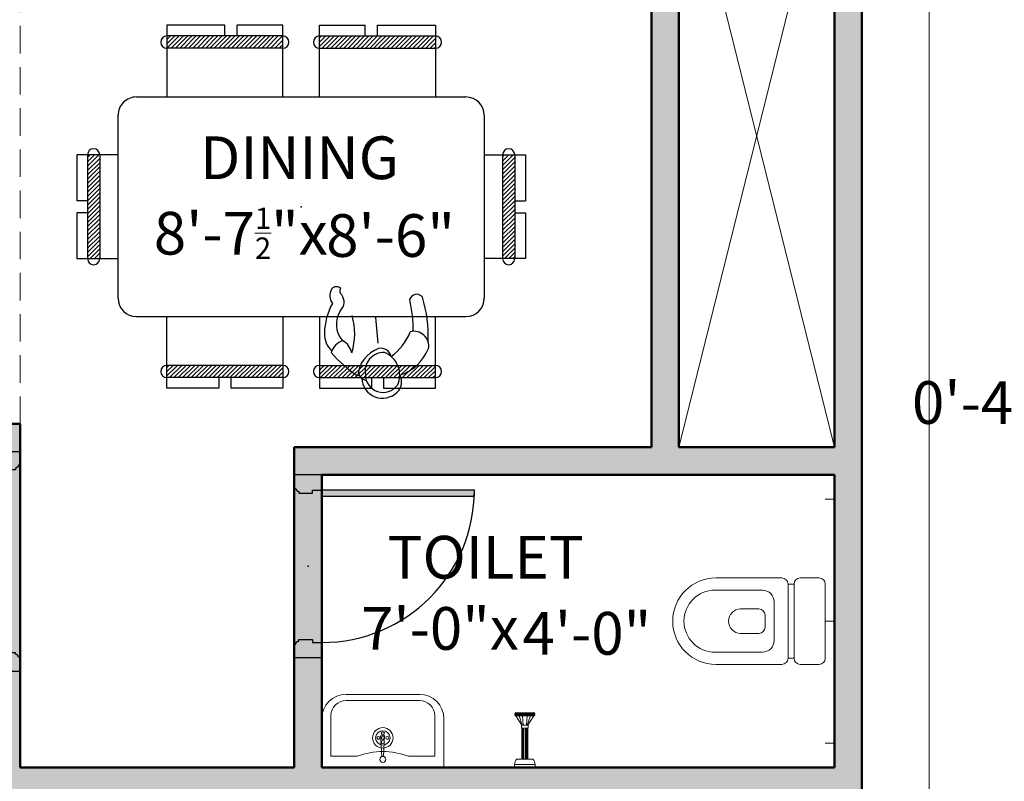
# Model space of a CAD drawing. Units: inches. Extents: x 4508 to 5907, y 877 to 1592.
# Tile 11 of 20: x 5392 to 5553, y 1049 to 1174. Entities that reach past the tile are written whole.
import ezdxf

# ---------------------------------------------------------------- set-up
doc = ezdxf.new("R2010")
doc.units = ezdxf.units.IN
doc.linetypes.add('DASHED', pattern=[0.75, 0.5, -0.25])
doc.layers.get('DEFPOINTS').update_dxf_attribs({"color": 8})
for name, color, linetype, lineweight in [('A-ANNO-DIMS', 2, 'Continuous', 18), ('A-DOOR', 4, 'Continuous', 25), ('A-FLOR-FIXT', 8, 'Continuous', 18), ('A-FLOR-OVHD', 5, 'DASHED', 18), ('A-FLOR-SHFT', 8, 'Continuous', 18), ('A-FURN', 24, 'Continuous', 18), ('A-WALL', 7, 'Continuous', 50), ('A-WALL-PATT', 8, 'Continuous', 13)]:
    doc.layers.add(name, color=color, linetype=linetype, lineweight=lineweight)
doc.layers.add('doors & windows', color=30, linetype='Continuous')
doc.layers.add('furniture', color=24, linetype='Continuous')
doc.styles.get("Standard").update_dxf_attribs({"font": 'arial.ttf'})
doc.dimstyles.new('details', dxfattribs={"dimtxt": 5, "dimasz": 2, "dimexe": 2, "dimexo": 3, "dimgap": 1, "dimtad": 0, "dimdec": 1, "dimzin": 0, "dimdsep": 46, "dimlunit": 4, "dimtxsty": 'Standard', "dimblk": 'ARCHTICK', "dimcen": 3, "dimclrd": 256, "dimclre": 256, "dimclrt": 256, "dimadec": 0, "dimazin": 0, "dimtfac": 0.5, "dimtdec": 1, "dimtofl": 0, "dimtmove": 0, "dimatfit": 3, "dimldrblk": 'CLOSEDBLANK', "dimfxl": 2, "dimtolj": 1, "dimtzin": 0, "dimlwd": -1, "dimlwe": -1, "dimarcsym": 0})
doc.dimstyles.new('text', dxfattribs={"dimtxt": 7, "dimasz": 0, "dimexe": 3, "dimexo": 3, "dimgap": 0, "dimtad": 1, "dimtih": 1, "dimtoh": 1, "dimzin": 3, "dimdsep": 46, "dimlunit": 4, "dimtxsty": 'Standard', "dimblk": 'CLOSEDBLANK', "dimcen": 3, "dimse1": 1, "dimse2": 1, "dimsd1": 1, "dimsd2": 1, "dimclrd": 256, "dimclre": 256, "dimclrt": 256, "dimadec": 0, "dimazin": 0, "dimtfac": 0.5, "dimtofl": 0, "dimtmove": 0, "dimatfit": 3, "dimfxl": 3, "dimtolj": 1, "dimtzin": 0, "dimlwd": -1, "dimlwe": -1, "dimarcsym": 0})
pattern_1 = [(45, (0, 0), (-0.3535534, 0.3535534), [])]

# ---------------------------------------------------------------- blocks, each defined once
blk = doc.blocks.new('*D94')
at = {"layer": 'DEFPOINTS', "color": 0, "transparency": 16777216}
for p in [(5391.9, 1143.25), (5495.4, 1139.55), (5391.9, 1134.58)]:
    blk.add_point(p, dxfattribs=at)
at = {"layer": 'A-ANNO-DIMS', "color": 0, "transparency": 16777216, "insert": (5428.13, 1144.63), "char_height": 7, "attachment_point": 5}
blk.add_mtext('\\A1;         DINING\\P8\'-7{\\H0.5x;\\S1/2;}"x', dxfattribs=at)
blk = doc.blocks.new('_ClosedBlank')
at = {"color": 0, "lineweight": -2}
for p, q in [((-1, 0.167), (0, 0)), ((-1, 0.167), (-1, -0.167)), ((0, 0), (-1, -0.167))]:
    blk.add_line(p, q, dxfattribs=at)
blk = doc.blocks.new('*D95')
at = {"layer": 'DEFPOINTS', "color": 0, "transparency": 16777216}
for p in [(5445.95, 1205.7), (5452.67, 1205.7), (5443.65, 1103.7)]:
    blk.add_point(p, dxfattribs=at)
at = {"layer": 'A-ANNO-DIMS', "color": 0, "transparency": 16777216, "insert": (5452.67, 1138.42), "char_height": 7, "attachment_point": 5}
blk.add_mtext('\\A1;8\'-6"', dxfattribs=at)
blk = doc.blocks.new('DT')
at = {"layer": 'furniture'}
h = blk.add_hatch(dxfattribs=at)
h.set_pattern_fill('ANSI31', color=256, scale=4, style=0)
h.set_pattern_definition(pattern_1)
h.paths.add_polyline_path([(-34, -8.5), (-32, -8.5), (-32, 8.5), (-34, 8.5)])
h.paths.add_polyline_path([(-2, 26), (-2, 28), (-21, 28), (-21, 26)])
h.paths.add_polyline_path([(23, 26), (23, 28), (4, 28), (4, 26)])
h.paths.add_polyline_path([(23, -28), (23, -26), (4, -26), (4, -28)])
h.paths.add_polyline_path([(-2, -28), (-2, -26), (-21, -26), (-21, -28)])
h = blk.add_hatch(dxfattribs=at)
h.set_pattern_fill('ANSI31', color=256, scale=4, style=0)
h.set_pattern_definition(pattern_1)
h.paths.add_polyline_path([(34, -8.5), (36, -8.5), (36, 8.5), (34, 8.5)])
at = {"layer": 'doors & windows'}
blk.add_line((-11.2, 18.15), (-11.59, 22.33), dxfattribs=at)
for centre, radius, start, end in [((-12.34, 27.96), 3.42, 2.8928, 134.5528), ((-13.21, 28.75), 2.25, 132.7993, 210.1219), ((-11.2, 27.56), 3.95, 155.2349, 248.5051), ((-12.43, 27.51), 2.91, 359.7942, 144.0351), ((-12.78, 20.33), 7.67, 108.0153, 157.5724), ((-12.53, 26.93), 3.05, 267.7788, 10.6507), ((-13.37, 28.03), 5.08, 289.2819, 356.6237), ((-9.72, 27.09), 1.31, 352.7443, 87.7525), ((-20.97, 8.73), 22.84, 41.647, 56.3067), ((-8.5, 17.23), 8.99, 125.6851, 158.6987), ((-12.08, 24.9), 1.7, 192.3382, 283.0231), ((-17.49, 22.83), 2.42, 170.002, 284.7527), ((2.64, 20.82), 10.42, 162.7002, 196.7262), ((-4.27, 24.65), 3.12, 193.5598, 239.9446), ((-6.9, 24.92), 3.16, 289.6374, 341.2911), ((-6.62, 20.83), 3.81, 358.2671, 46.939), ((1.32, 21.08), 21.14, 177.1977, 197.248), ((-8.79, 19.27), 4.03, 325.4363, 41.8446), ((6.61, 20.49), 23.98, 180.1725, 192.6992), ((-13.17, 20.91), 10.36, 330.7562, 358.8997), ((-4.02, 15.59), 2.01, 136.0875, 215.1077), ((-17.93, 15.53), 1.19, 217.214, 345.0614), ((-5.73, 14.57), 2.04, 328.4119, 38.6474), ((-5.98, 13.86), 0.655, 315.9836, 61.7947), ((-4.79, 14.1), 0.998, 224.0636, 323.687)]:
    blk.add_arc(centre, radius, start, end, dxfattribs=at)
at = {"layer": 'furniture'}
for p, q in [((-21, 29.75), (-21, 18)), ((-12.5, 29.75), (-21, 29.75)), ((-12.5, 28), (-12.5, 29.75)), ((-10.5, 28), (-10.5, 29.75)), ((-2, 29.75), (-10.5, 29.75)), ((-2, 18), (-2, 29.75)), ((4, 18), (4, 29.75)), ((4, 29.75), (12.5, 29.75)), ((12.5, 28), (12.5, 29.75)), ((14.5, 28), (14.5, 29.75)), ((14.5, 29.75), (23, 29.75)), ((23, 29.75), (23, 18)), ((-2, 28), (-21, 28)), ((4, 28), (23, 28)), ((-2, 26), (-21, 26)), ((4, 26), (23, 26)), ((28, 18), (-26, 18)), ((-29, -15), (-29, 15)), ((31, 15), (31, -15)), ((-35.75, 1), (-35.75, 8.5)), ((-35.75, 8.5), (-29, 8.5)), ((-34, -8.5), (-34, 8.5)), ((-32, -8.5), (-32, 8.5)), ((37.75, 8.5), (31, 8.5)), ((34, -8.5), (34, 8.5)), ((36, -8.5), (36, 8.5)), ((37.75, 1), (37.75, 8.5)), ((-34, 1), (-35.75, 1)), ((36, 1), (37.75, 1)), ((-34, -1), (-35.75, -1)), ((-35.75, -8.5), (-35.75, -1)), ((36, -1), (37.75, -1)), ((37.75, -8.5), (37.75, -1)), ((-29, -8.5), (-35.75, -8.5)), ((31, -8.5), (37.75, -8.5)), ((28, -18), (-26, -18)), ((-21, -29.75), (-21, -18)), ((-2, -18), (-2, -29.75)), ((4, -18), (4, -29.75)), ((23, -29.75), (23, -18)), ((-2, -26), (-21, -26)), ((4, -26), (23, -26)), ((-2, -28), (-21, -28)), ((-11.5, -28), (-11.5, -29.75)), ((-9.5, -28), (-9.5, -29.75)), ((4, -28), (23, -28)), ((11.5, -28), (11.5, -29.75)), ((13.5, -28), (13.5, -29.75)), ((-11.5, -29.75), (-21, -29.75)), ((-2, -29.75), (-9.5, -29.75)), ((4, -29.75), (11.5, -29.75)), ((13.5, -29.75), (23, -29.75))]:
    blk.add_line(p, q, dxfattribs=at)
for centre, radius, start, end in [((-21, 27), 1, 90, 270), ((-2, 27), 1, 270, 90), ((4, 27), 1, 90, 270), ((23, 27), 1, 270, 90), ((-26, 15), 3, 90, 180), ((28, 15), 3, 0, 90), ((-33, 8.5), 1, 0, 180), ((35, 8.5), 1, 0, 180), ((-33, -8.5), 1, 180, 0), ((35, -8.5), 1, 180, 0), ((-26, -15), 3, 180, 270), ((28, -15), 3, 270, 0), ((-21, -27), 1, 90, 270), ((-2, -27), 1, 270, 90), ((4, -27), 1, 90, 270), ((23, -27), 1, 270, 90)]:
    blk.add_arc(centre, radius, start, end, dxfattribs=at)
blk.add_point((1, 0), dxfattribs=at)
blk = doc.blocks.new('D1')
at = {"layer": 'doors & windows'}
h = blk.add_hatch(dxfattribs=at)
h.set_pattern_fill('DOTS', color=256, scale=2, angle=180, style=0)
h.set_pattern_definition([(180, (-2e-12, -4), (-0.0625, -0.125), [0, -0.125])])
h.paths.add_polyline_path([(2.5, 0), (3.5, 0), (3.5, 30.98, 0.008066), (2.5, 31)])
h = blk.add_hatch(dxfattribs=at)
h.set_pattern_fill('DOTS', color=256, scale=2, angle=180, style=0)
h.set_pattern_definition([(180, (0, -0.5), (-0.0625, -0.125), [0, -0.125])])
h.paths.add_polyline_path([(0, -4.5), (2.25, -4.5), (2.25, -4.25, 0.403966), (2.75, -3.75), (3, -3.75), (3, -1.5), (2.5, -1.5), (2.5, 0), (0, 0)])
h.paths.add_polyline_path([(36, -4.5), (36, 0), (33.5, 0), (33.5, -1.5), (33, -1.5), (33, -3.75), (33.25, -3.75, 0.403966), (33.75, -4.25), (33.75, -4.5)])
for p, q in [((0, 0), (0, -4.5)), ((36, 0), (36, -4.5))]:
    blk.add_line(p, q)
blk.add_lwpolyline([(3.5, 0), (3.5, 31), (2.5, 31), (2.5, 0)], close=True, dxfattribs=at)
for points in [[(3, -3.75), (3, -1.5), (2.5, -1.5), (2.5, 0), (0, 0)], [(33, -3.75), (33, -1.5), (33.5, -1.5), (33.5, 0), (36, 0)], [(0, -4.5), (2.25, -4.5)], [(36, -4.5), (33.75, -4.5)]]:
    blk.add_lwpolyline(points, dxfattribs=at)
for points in [[(2.25, -4.5), (2.25, -4.25, 0.403966), (2.75, -3.75), (3, -3.75)], [(33.75, -4.5), (33.75, -4.25, -0.403966), (33.25, -3.75), (33, -3.75)]]:
    blk.add_lwpolyline(points, format="xyb", dxfattribs=at)
at = {"layer": 'doors & windows', "ltscale": 6}
blk.add_arc((2.5, 0), 31, 0, 90, dxfattribs=at)
at = {"layer": 'doors & windows'}
blk.add_point((18, -2.75), dxfattribs=at)
blk = doc.blocks.new('D2')
at = {"layer": 'doors & windows'}
h = blk.add_hatch(dxfattribs=at)
h.set_pattern_fill('DOTS', color=256, scale=2, angle=180, style=0)
h.set_pattern_definition([(180, (0, -4), (-0.0625, -0.125), [0, -0.125])])
h.paths.add_polyline_path([(2.5, 0), (3.5, 0), (3.5, 24.98, 0.010003), (2.5, 25)])
h = blk.add_hatch(dxfattribs=at)
h.set_pattern_fill('DOTS', color=256, scale=2, angle=180, style=0)
h.set_pattern_definition([(180, (0, 0), (-0.0625, -0.125), [0, -0.125])])
edge = h.paths.add_edge_path()
edge.add_line((27.5, 0), (27.5, -1.5))
edge.add_line((27.5, -1.5), (27, -1.5))
edge.add_line((27, -1.5), (27, -3.75))
edge.add_line((27, -3.75), (27.25, -3.75))
edge.add_arc((27.76, -3.74), 0.509, 181.0059, 268.9941)
edge.add_line((27.75, -4.25), (27.75, -4.5))
edge.add_line((27.75, -4.5), (30, -4.5))
edge.add_line((30, -4.5), (30, 0))
edge.add_line((30, 0), (27.5, 0))
edge = h.paths.add_edge_path()
edge.add_line((2.5, -1.5), (2.5, 0))
edge.add_line((2.5, 0), (0, 0))
edge.add_line((0, 0), (0, -4.5))
edge.add_line((0, -4.5), (2.25, -4.5))
edge.add_line((2.25, -4.5), (2.25, -4.25))
edge.add_arc((2.24, -3.74), 0.509, 271.0059, 358.9941)
edge.add_line((2.75, -3.75), (3, -3.75))
edge.add_line((3, -3.75), (3, -1.5))
edge.add_line((3, -1.5), (2.5, -1.5))
for p, q in [((0, 0), (0, -4.5)), ((30, 0), (30, -4.5))]:
    blk.add_line(p, q)
blk.add_lwpolyline([(3.5, 0), (3.5, 25), (2.5, 25), (2.5, 0)], close=True, dxfattribs=at)
for points in [[(3, -3.75), (3, -1.5), (2.5, -1.5), (2.5, 0), (0, 0)], [(27, -3.75), (27, -1.5), (27.5, -1.5), (27.5, 0), (30, 0)], [(0, -4.5), (2.25, -4.5)], [(30, -4.5), (27.75, -4.5)]]:
    blk.add_lwpolyline(points, dxfattribs=at)
for points in [[(2.25, -4.5), (2.25, -4.25, 0.403966), (2.75, -3.75), (3, -3.75)], [(27.75, -4.5), (27.75, -4.25, -0.403966), (27.25, -3.75), (27, -3.75)]]:
    blk.add_lwpolyline(points, format="xyb", dxfattribs=at)
at = {"layer": 'doors & windows', "ltscale": 6}
blk.add_arc((2.5, 0), 25, 0, 90, dxfattribs=at)
at = {"layer": 'doors & windows'}
blk.add_point((15, -2.25), dxfattribs=at)
blk = doc.blocks.new('commode')
for p, q in [((-7.09, 19.41), (-7.09, 8.61)), ((-5.09, 11.81), (-5.09, 19.57)), ((5.09, 11.81), (5.09, 19.57)), ((7.09, 19.41), (7.09, 8.61)), ((-2, 12.37), (-2, 15.37)), ((2, 12.37), (2, 15.37)), ((-1, 11.37), (1, 11.37)), ((-3.15, 9.87), (3.15, 9.87)), ((-6.09, 7.61), (6.09, 7.61)), ((-6.09, 6.61), (-6.09, 7.61)), ((-6.09, 6.61), (6.09, 6.61)), ((6.09, 7.61), (6.09, 6.61)), ((-7.09, 2.5), (-7.09, 5.61)), ((7.09, 2.5), (7.09, 5.61)), ((-20, 1.5), (-20, 0)), ((-6.09, 1.5), (6.09, 1.5)), ((0, 1.5), (0, 0)), ((20, 1.5), (20, 0))]:
    blk.add_line(p, q)
for centre, radius, start, end in [((0, 19.41), 7.09, 0, 180), ((0, 19.57), 5.09, 0, 180), ((0, 15.37), 2, 0, 180), ((-3.15, 11.81), 1.94, 180, 270), ((-1, 12.37), 1, 180, 270), ((1, 12.37), 1, 270, 0), ((3.15, 11.81), 1.94, 270, 0), ((-6.09, 8.61), 1, 180, 270), ((6.09, 8.61), 1, 270, 0), ((-6.09, 5.61), 1, 90, 180), ((6.09, 5.61), 1, 0, 90), ((-6.09, 2.5), 1, 180, 270), ((6.09, 2.5), 1, 270, 0)]:
    blk.add_arc(centre, radius, start, end)
blk = doc.blocks.new('wash basin 1')
for p, q in [((0, 10), (-8, 10)), ((0, 10), (0, -10)), ((-8.5, 8.5), (-1.85, 8.5)), ((-1.85, 8.5), (-1.85, 4.19)), ((-12, 6), (-12, -6)), ((-11, 6), (-11, -6)), ((-1.85, -8.5), (-1.85, -4.19)), ((-8.5, -8.5), (-1.85, -8.5)), ((0, -10), (-8, -10))]:
    blk.add_line(p, q)
blk.add_lwpolyline([(-1.83, 0.11), (-5.25, 0.25), (-5.23, -0.38), (-1.8, -0.19)])
for centre, radius in [((-4.87, 0), 1.68), ((-4.87, 0), 1.18), ((-5.63, 0), 0.25), ((-4.87, 0.75), 0.25), ((-4.87, 0), 0.25), ((-4.19, 0), 0.25), ((-1.34, 0), 0.5), ((-4.87, -0.72), 0.25)]:
    blk.add_circle(centre, radius)
for centre, radius, start, end in [((-8, 6), 4, 90, 180), ((-8.5, 6), 2.5, 90, 180), ((8.89, 0), 11.53, 158.7059, 201.2941), ((-8, -6), 4, 180, 270), ((-8.5, -6), 2.5, 180, 270)]:
    blk.add_arc(centre, radius, start, end)
blk = doc.blocks.new('tap & shower')
for p, q in [((1.71, 0), (-1.71, 0)), ((-1.71, 0), (-1.71, -0.5)), ((1.71, 0), (1.71, -0.5)), ((1.71, -0.5), (-1.71, -0.5)), ((1.31, -1.4), (-1.31, -1.4)), ((-0.5, -6.44), (-0.5, -1.4)), ((-0.42, -6.44), (-0.42, -1.4)), ((-0.32, -0.5), (0.32, -0.5)), ((-0.3, -6.44), (-0.3, -1.4)), ((-0.14, -6.44), (-0.14, -1.4)), ((0.14, -6.44), (0.14, -1.4)), ((0.3, -6.44), (0.3, -1.4)), ((0.42, -6.44), (0.42, -1.4)), ((0.5, -6.44), (0.5, -1.4)), ((-0.56, -6.44), (0.56, -6.44)), ((-0.56, -6.98), (-0.56, -6.44)), ((0.56, -6.98), (0.56, -6.44)), ((-1.48, -8.46), (-0.47, -6.98)), ((-0.41, -6.98), (-0.94, -8.46)), ((-0.56, -6.98), (0.56, -6.98)), ((-0.29, -6.98), (-0.4, -8.46)), ((0.29, -6.98), (0.4, -8.46)), ((0.41, -6.98), (0.94, -8.46)), ((1.48, -8.46), (0.47, -6.98)), ((-1.62, -8.87), (-1.62, -8.6)), ((-1.48, -8.46), (1.48, -8.46)), ((-1.48, -9), (-1.48, -8.46)), ((-1.48, -9), (1.48, -9)), ((-1.43, -9), (-1.43, -8.46)), ((-1.37, -9), (-1.37, -8.46)), ((-1.32, -9), (-1.32, -8.46)), ((-1.27, -9), (-1.27, -8.46)), ((-1.21, -9), (-1.21, -8.46)), ((-1.16, -9), (-1.16, -8.46)), ((-1.1, -9), (-1.1, -8.46)), ((-1.05, -9), (-1.05, -8.46)), ((-1, -9), (-1, -8.46)), ((-0.94, -9), (-0.94, -8.46)), ((-0.89, -9), (-0.89, -8.46)), ((-0.84, -9), (-0.84, -8.46)), ((-0.78, -9), (-0.78, -8.46)), ((-0.73, -9), (-0.73, -8.46)), ((-0.67, -9), (-0.67, -8.46)), ((-0.62, -9), (-0.62, -8.46)), ((-0.57, -9), (-0.57, -8.46)), ((-0.51, -9), (-0.51, -8.46)), ((-0.46, -9), (-0.46, -8.46)), ((-0.4, -9), (-0.4, -8.46)), ((-0.35, -9), (-0.35, -8.46)), ((-0.3, -9), (-0.3, -8.46)), ((-0.24, -9), (-0.24, -8.46)), ((-0.19, -9), (-0.19, -8.46)), ((-0.13, -9), (-0.13, -8.46)), ((-0.08, -9), (-0.08, -8.46)), ((-0.03, -9), (-0.03, -8.46)), ((0.03, -9), (0.03, -8.46)), ((0.08, -9), (0.08, -8.46)), ((0.13, -9), (0.13, -8.46)), ((0.19, -9), (0.19, -8.46)), ((0.24, -9), (0.24, -8.46)), ((0.3, -9), (0.3, -8.46)), ((0.35, -9), (0.35, -8.46)), ((0.4, -9), (0.4, -8.46)), ((0.46, -9), (0.46, -8.46)), ((0.51, -9), (0.51, -8.46)), ((0.57, -9), (0.57, -8.46)), ((0.62, -9), (0.62, -8.46)), ((0.67, -9), (0.67, -8.46)), ((0.73, -9), (0.73, -8.46)), ((0.78, -9), (0.78, -8.46)), ((0.84, -9), (0.84, -8.46)), ((0.89, -9), (0.89, -8.46)), ((0.94, -9), (0.94, -8.46)), ((1, -9), (1, -8.46)), ((1.05, -9), (1.05, -8.46)), ((1.1, -9), (1.1, -8.46)), ((1.16, -9), (1.16, -8.46)), ((1.21, -9), (1.21, -8.46)), ((1.27, -9), (1.27, -8.46)), ((1.32, -9), (1.32, -8.46)), ((1.37, -9), (1.37, -8.46)), ((1.43, -9), (1.43, -8.46)), ((1.48, -9), (1.48, -8.46)), ((1.62, -8.87), (1.62, -8.6))]:
    blk.add_line(p, q)
for centre, radius, start, end in [((-0.02, -0.29), 1.7, 187.1825, 220.9028), ((0.02, -0.29), 1.7, 319.0972, 352.8175), ((-1.48, -8.6), 0.135, 90, 180), ((-1.48, -8.87), 0.135, 180, 270), ((1.48, -8.6), 0.135, 0, 90), ((1.48, -8.87), 0.135, 270, 0)]:
    blk.add_arc(centre, radius, start, end)
blk = doc.blocks.new('*D107')
at = {"layer": 'DEFPOINTS', "color": 0, "transparency": 16777216}
for p in [(5525.4, 1070.38), (5441.4, 1069.2), (5525.4, 1067.89)]:
    blk.add_point(p, dxfattribs=at)
at = {"layer": 'A-ANNO-DIMS', "color": 0, "transparency": 16777216, "insert": (5460.77, 1079.85), "char_height": 7, "attachment_point": 5}
blk.add_mtext('\\A1;       TOILET\\P7\'-0"x', dxfattribs=at)
blk = doc.blocks.new('*D108')
at = {"layer": 'DEFPOINTS', "color": 0, "transparency": 16777216}
for p in [(5480.14, 1099.2), (5483.4, 1051.2), (5484.84, 1051.2)]:
    blk.add_point(p, dxfattribs=at)
at = {"layer": 'A-ANNO-DIMS', "color": 0, "transparency": 16777216, "insert": (5484.84, 1073.21), "char_height": 7, "attachment_point": 5}
blk.add_mtext('\\A1;4\'-0"', dxfattribs=at)
blk = doc.blocks.new('_ArchTick')
at = {"color": 0, "linetype": 'ByBlock', "const_width": 0.15}
blk.add_lwpolyline([(-0.5, -0.5), (0.5, 0.5)], dxfattribs=at)
blk = doc.blocks.new('*D113')
at = {"layer": 'A-ANNO-DIMS', "color": 0, "transparency": 16777216}
for p, q in [((5532.9, 1574.7), (5542.92, 1574.7)), ((5540.92, 1574.7), (5540.92, 1255.95)), ((5540.92, 926.7), (5540.92, 1245.46)), ((5532.9, 926.7), (5542.92, 926.7))]:
    blk.add_line(p, q, dxfattribs=at)
at = {"layer": 'DEFPOINTS', "color": 0, "transparency": 16777216}
for p in [(5529.9, 1574.7), (5540.92, 1574.7), (5529.9, 926.7)]:
    blk.add_point(p, dxfattribs=at)
at = {"layer": 'A-ANNO-DIMS', "color": 0, "transparency": 16777216, "xscale": 2, "yscale": 2, "zscale": 2}
for p, rotation in [((5540.92, 1574.7), 90), ((5540.92, 926.7), 270)]:
    blk.add_blockref('_ArchTick', p, dxfattribs=dict(at, rotation=rotation))
at = {"layer": 'A-ANNO-DIMS', "color": 0, "transparency": 16777216, "insert": (5540.92, 1250.7), "char_height": 5, "attachment_point": 5, "rotation": 90}
blk.add_mtext("\\A1;54'", dxfattribs=at)
blk = doc.blocks.new('*D193')
at = {"layer": 'DEFPOINTS', "color": 0, "transparency": 16777216}
for p in [(5539.44, 1111.92), (5580.63, 1111.92), (5580.65, 1107.42)]:
    blk.add_point(p, dxfattribs=at)
at = {"layer": 'A-ANNO-DIMS', "transparency": 16777216, "insert": (5556.9, 1111.04), "char_height": 7, "attachment_point": 5}
blk.add_mtext('\\A1;0\'-4 1/2"', dxfattribs=at)

msp = doc.modelspace()

# ---------------------------------------------------------------- hatches: boundary and pattern name
at = {"layer": 'A-WALL-PATT'}
h = msp.add_hatch(color=256, dxfattribs=at)
h.dxf.hatch_style = 1
h.paths.add_polyline_path([(5529.903, 1303.204), (5388.02, 1303.204), (5388.02, 1294.204), (5391.903, 1294.204), (5391.903, 1205.704), (5396.403, 1205.704), (5396.403, 1294.204), (5489.403, 1294.204), (5489.403, 1256.139), (5493.903, 1256.139), (5493.903, 1294.204), (5529.903, 1294.204)], flags=17)
h.paths.add_polyline_path([(5346.02, 1303.204), (5322.903, 1303.204), (5322.903, 1321.388), (5313.903, 1321.388), (5313.903, 1303.204), (5259.903, 1303.204), (5259.903, 1381.204), (5313.903, 1381.204), (5313.903, 1359.674), (5322.903, 1359.674), (5322.903, 1381.204), (5338.979, 1381.204), (5338.979, 1390.204), (5331.903, 1390.204), (5331.903, 1442.704), (5255.403, 1442.704), (5255.403, 1570.204), (5387.403, 1570.204), (5387.403, 1541.271), (5391.903, 1541.271), (5391.903, 1570.204), (5483.403, 1570.204), (5483.403, 1498.204), (5391.903, 1498.204), (5391.903, 1509.559), (5387.403, 1509.559), (5387.403, 1390.204), (5380.979, 1390.204), (5380.979, 1381.204), (5387.403, 1381.204), (5529.903, 1381.204), (5529.903, 1498.204), (5487.903, 1498.204), (5487.903, 1570.204), (5529.903, 1570.204), (5529.903, 1574.704), (5250.903, 1574.704), (5250.903, 991.204), (5310.903, 991.204), (5310.903, 926.704), (5529.903, 926.704), (5529.903, 1210.204), (5525.403, 1210.204), (5525.403, 1103.704), (5499.903, 1103.704), (5499.903, 1210.204), (5493.903, 1210.204), (5493.903, 1256.139), (5489.403, 1256.139), (5489.403, 1210.204), (5461.584, 1210.204), (5461.584, 1205.704), (5495.403, 1205.704), (5495.403, 1103.704), (5436.903, 1103.704), (5436.903, 1051.204), (5391.954, 1051.204), (5391.954, 1103.03), (5391.954, 1107.53), (5255.403, 1108.204), (5255.403, 1294.204), (5346.02, 1294.204)])
h.paths.add_polyline_path([(5255.403, 1390.204), (5255.403, 1398.204), (5255.403, 1438.204), (5257.903, 1438.204), (5258.903, 1438.204), (5327.403, 1438.204), (5327.403, 1390.204), (5325.903, 1390.204)], flags=16)
h.paths.add_polyline_path([(5288.757, 1390.704), (5288.757, 1390.204), (5292.173, 1390.204), (5292.173, 1390.704)], flags=0)
h.paths.add_polyline_path([(5289.965, 1391.606), (5289.965, 1396.645), (5289.903, 1396.645), (5289.903, 1397.319), (5288.849, 1398.862), (5288.849, 1398.8), (5288.983, 1398.748), (5288.983, 1399.204), (5289.091, 1399.204), (5292.081, 1399.204), (5292.081, 1398.665), (5291.946, 1398.665), (5291.027, 1397.319), (5291.027, 1396.645), (5290.965, 1396.645), (5290.965, 1391.606)], flags=0)
h.paths.add_polyline_path([(5288.849, 1399.069, 2.6374395), (5289.056, 1398.835), (5289.117, 1399.087, 0.9346155)], flags=0)
h.paths.add_polyline_path([(5290.061, 1398.665), (5290.061, 1399.204), (5290.038, 1398.975)], flags=0)
h.paths.add_polyline_path([(5291.946, 1398.934, -1), (5291.946, 1398.665)], flags=0)
h.paths.add_polyline_path([(5289.414, 1398.967), (5289.414, 1399.204), (5289.63, 1399.204), (5289.63, 1398.363), (5290.051, 1397.184), (5290.76, 1397.184), (5290.869, 1398.665), (5290.869, 1399.204), (5290.815, 1398.665), (5290.815, 1399.204), (5291.462, 1399.204), (5291.462, 1398.816), (5290.879, 1397.184), (5290.051, 1397.184)], flags=0)
h.paths.add_polyline_path([(5273.903, 1392.056), (5269.591, 1392.056, 0.0901028), (5265.544, 1392.842), (5265.511, 1392.034, -0.3516542), (5265.903, 1391.546, -1), (5264.903, 1391.546, -0.3042165), (5265.213, 1392.008), (5265.167, 1392.84, 0.0880132), (5261.215, 1392.056), (5256.903, 1392.056), (5256.903, 1398.704, -0.4142136), (5259.403, 1401.204), (5271.403, 1401.204, -0.4142136), (5273.903, 1398.704)], flags=0)
h.paths.add_polyline_path([(5263.726, 1395.073, -1), (5267.08, 1395.073, -1)], flags=0)
h.paths.add_polyline_path([(5264.434, 1395.073, -0.695521), (5265.153, 1395.073, -1.1408699), (5265.403, 1395.585, -0.7522125), (5265.403, 1396.25, 0.3674806)], flags=0)
h.paths.add_polyline_path([(5265.153, 1394.399, -1), (5265.653, 1394.399, -1)], flags=0)
h.paths.add_polyline_path([(5265.905, 1395.077, -1), (5266.405, 1395.077, -1)], flags=0)
h.paths.add_polyline_path([(5307.994, 1403.113, -1), (5307.994, 1417.295), (5318.794, 1417.295, -0.4142136), (5319.794, 1416.295), (5320.794, 1416.295, -0.4142136), (5321.794, 1417.295), (5324.903, 1417.295, -0.4142136), (5325.903, 1416.295), (5325.903, 1404.113, -0.4142136), (5324.903, 1403.113), (5321.794, 1403.113, -0.4142136), (5320.794, 1404.113), (5319.794, 1404.113, -0.4142136), (5318.794, 1403.113)], flags=0)
h.paths.add_polyline_path([(5307.836, 1405.113, -1), (5307.836, 1415.295), (5315.591, 1415.295, -0.4142136), (5317.532, 1413.353), (5317.532, 1407.054, -0.4142136), (5315.591, 1405.113)], flags=0)
h.paths.add_polyline_path([(5312.032, 1408.204, -1), (5312.032, 1412.204), (5315.032, 1412.204, -0.4142136), (5316.032, 1411.204), (5316.032, 1409.204, -0.4142136), (5315.032, 1408.204)], flags=0)
h.paths.add_polyline_path([(5391.903, 1385.704), (5391.903, 1493.704), (5525.403, 1493.704), (5525.403, 1385.704)], flags=16)
h.paths.add_polyline_path([(5422.641, 1390.704), (5422.641, 1465.704, -0.9426302), (5422.641, 1467.704), (5494.547, 1467.704, -1), (5494.665, 1465.704), (5494.665, 1390.704, -0.9426302), (5494.665, 1388.704), (5422.759, 1388.704, -1)], flags=0)
h.paths.add_polyline_path([(5427.52, 1395.749, -0.0238564), (5427.614, 1403.949, 0.0884332), (5427.476, 1405.056, 0.0506693), (5427.273, 1405.463, -0.8716827), (5427.713, 1405.835, 0.0268855), (5431.815, 1405.361, 0.0306964), (5436.289, 1405.361, -0.0263641), (5445.798, 1405.259, 0.075811), (5450.408, 1405.53, 0.0687062), (5454.457, 1405.903, -1.0086747), (5454.781, 1405.482, 0.0692081), (5454.389, 1400.959, -0.0519468), (5454.356, 1394.996, 0.1195012), (5454.627, 1392.895, 0.0143508), (5454.796, 1392.489, -0.6962059), (5454.42, 1392.118, 0.1574808), (5448.747, 1392.794, -0.025536), (5432.749, 1392.774, 0.0920085), (5427.781, 1392.048, -0.9384848), (5427.137, 1392.455, 0.0063894), (5427.314, 1392.79, 0.0472995)], flags=0)
h.paths.add_polyline_path([(5426.125, 1411.372, 0.0617649), (5428.641, 1412.201), (5428.641, 1465.704), (5488.665, 1465.704), (5488.665, 1412.363, 0.2363822), (5467.6, 1412.052, -0.2252042)], flags=0)
h.paths.add_polyline_path([(5391.903, 1490.204), (5391.903, 1491.204), (5422.903, 1491.204), (5422.903, 1490.204)], flags=0)
h.paths.add_polyline_path([(5462.545, 1392.771, 0.1270318), (5462.866, 1394.996, -0.0519468), (5462.832, 1400.959, 0.0692081), (5462.441, 1405.482, -1.0086747), (5462.765, 1405.903, 0.0857004), (5471.424, 1405.259, -0.0263641), (5480.932, 1405.361, 0.0306964), (5485.407, 1405.361, 0.0268855), (5489.509, 1405.835, -0.8716827), (5489.949, 1405.463, 0.0506693), (5489.746, 1405.056, 0.0884332), (5489.608, 1403.949, -0.0238564), (5489.702, 1395.749, 0.0472995), (5489.908, 1392.79, 0.0063894), (5490.085, 1392.455, -0.9384848), (5489.441, 1392.048, 0.0920085), (5484.473, 1392.774, -0.025536), (5468.475, 1392.794, 0.1574808), (5462.802, 1392.118, -0.6962059), (5462.426, 1392.489, 0.0100173), (5462.546, 1392.771)], flags=0)
h.paths.add_polyline_path([(5387.454, 1103.03), (5387.454, 1100.53), (5387.454, 1099.53), (5387.454, 995.03), (5387.454, 991.204), (5391.954, 991.204), (5391.954, 1046.704), (5525.403, 1046.704), (5525.403, 931.182), (5391.954, 930.53), (5391.954, 960.53), (5387.454, 960.53), (5387.454, 930.53), (5315.403, 930.53), (5315.403, 991.204), (5323.403, 991.204), (5387.454, 991.204), (5387.454, 995.03), (5255.403, 995.704), (5255.403, 1103.704)], flags=16)
h.paths.add_polyline_path([(5379.264, 1062.889), (5379.264, 1060.156), (5385.764, 1061.889, -0.4526903), (5385.764, 1059.889), (5379.264, 1059.889), (5379.264, 1055.156), (5385.764, 1056.889, -0.4526903), (5385.764, 1054.889), (5379.264, 1054.889), (5379.264, 1050.156), (5385.764, 1051.889, -0.4526903), (5385.764, 1049.889), (5379.264, 1049.889), (5379.264, 1010.156), (5385.764, 1011.889, -0.4526903), (5385.764, 1009.889), (5379.264, 1009.889), (5379.264, 1005.156), (5385.764, 1006.889, -0.4526903), (5385.764, 1004.889), (5379.264, 1004.889), (5379.264, 1000.156), (5385.764, 1001.889, -0.4526903), (5385.764, 999.889), (5378.264, 999.889), (5370.764, 997.889, -0.6674863), (5370.764, 999.889), (5377.264, 999.889), (5377.264, 1004.623), (5370.764, 1002.889, -0.6674863), (5370.764, 1004.889), (5377.264, 1004.889), (5377.264, 1009.623), (5370.764, 1007.889, -0.6674863), (5370.764, 1009.889), (5377.264, 1009.889), (5377.264, 1049.623), (5370.764, 1047.889, -0.6674863), (5370.764, 1049.889), (5377.264, 1049.889), (5377.264, 1054.623), (5370.764, 1052.889, -0.6674863), (5370.764, 1054.889), (5377.264, 1054.889), (5377.264, 1059.623), (5370.764, 1057.889, -0.6674863), (5370.764, 1059.889), (5377.264, 1059.889), (5377.264, 1062.889)], flags=0)
h.paths.add_polyline_path([(5287.641, 1000.704), (5359.665, 1000.704), (5359.665, 1018.212, 0.3202856), (5332.6, 1022.052, -0.246494), (5287.641, 1023.128)], flags=0)
h.paths.add_polyline_path([(5359.547, 1077.704, -1), (5359.665, 1075.704), (5353.665, 1075.704), (5353.665, 1063.704), (5293.641, 1063.704), (5293.641, 1075.704), (5287.759, 1075.704, -1), (5287.641, 1077.704)], flags=0)
h.paths.add_polyline_path([(5441.403, 1099.204), (5525.403, 1099.204), (5525.403, 1051.204), (5441.403, 1051.204), (5441.403, 1059.204)], flags=16)
h.paths.add_polyline_path([(5441.403, 1096.704), (5466.403, 1096.704), (5466.403, 1095.704), (5441.403, 1095.704)], flags=0)
h.paths.add_polyline_path([(5445.403, 1062.204), (5457.403, 1062.204, -0.4142136), (5459.903, 1059.704), (5459.903, 1053.056), (5455.591, 1053.056, 0.0901028), (5451.544, 1053.842), (5451.511, 1053.034, -0.3516542), (5451.903, 1052.546, -1), (5450.903, 1052.546, -0.3042165), (5451.213, 1053.008), (5451.167, 1053.84, 0.0880132), (5447.215, 1053.056), (5442.903, 1053.056), (5442.903, 1059.704, -0.4142136)], flags=0)
h.paths.add_polyline_path([(5453.08, 1056.073, -1), (5449.726, 1056.073, -1)], flags=0)
h.paths.add_polyline_path([(5292.713, 1015.835, 0.0268855), (5296.815, 1015.361, 0.0306964), (5301.289, 1015.361, -0.0263641), (5310.798, 1015.259, 0.075811), (5315.408, 1015.53, 0.0687062), (5319.457, 1015.903, -1.0086747), (5319.781, 1015.482, 0.0692081), (5319.389, 1010.959, -0.0519468), (5319.356, 1004.996, 0.1195012), (5319.627, 1002.895, 0.0143508), (5319.796, 1002.489, -0.6962059), (5319.42, 1002.118, 0.1574808), (5313.747, 1002.794, -0.025536), (5297.749, 1002.774, 0.0920085), (5292.781, 1002.048, -0.9384848), (5292.137, 1002.455, 0.0063894), (5292.314, 1002.79, 0.0472995), (5292.52, 1005.749, -0.0238564), (5292.614, 1013.949, 0.0884332), (5292.476, 1015.056, 0.0506693), (5292.273, 1015.463, -0.8716827)], flags=0)
h.paths.add_polyline_path([(5450.434, 1056.073, -0.695521), (5451.153, 1056.073, -1.1408699), (5451.403, 1056.585, -0.7522125), (5451.403, 1057.25, 0.3674806)], flags=0)
h.paths.add_polyline_path([(5327.765, 1015.903, 0.0857004), (5336.424, 1015.259, -0.0263641), (5345.932, 1015.361, 0.0306964), (5350.407, 1015.361, 0.0268855), (5354.509, 1015.835, -0.8716827), (5354.949, 1015.463, 0.0506693), (5354.746, 1015.056, 0.0884332), (5354.608, 1013.949, -0.0238564), (5354.702, 1005.749, 0.0472995), (5354.908, 1002.79, 0.0063894), (5355.085, 1002.455, -0.9384848), (5354.441, 1002.048, 0.0920085), (5349.473, 1002.774, -0.025536), (5333.475, 1002.794, 0.1574808), (5327.802, 1002.118, -0.6962059), (5327.426, 1002.489, 0.0100173), (5327.546, 1002.771), (5327.545, 1002.771, 0.1270318), (5327.866, 1004.996, -0.0519468), (5327.832, 1010.959, 0.0692081), (5327.441, 1015.482, -1.0086747)], flags=0)
h.paths.add_polyline_path([(5452.405, 1056.077, -1), (5451.905, 1056.077, -1)], flags=0)
h.paths.add_polyline_path([(5451.653, 1055.399, -1), (5451.153, 1055.399, -1)], flags=0)
h.paths.add_polyline_path([(5472.958, 1051.704), (5472.958, 1051.204), (5476.374, 1051.204), (5476.374, 1051.704)], flags=0)
h.paths.add_polyline_path([(5476.282, 1060.204), (5476.282, 1059.665), (5476.147, 1059.665), (5475.228, 1058.319), (5475.228, 1057.645), (5475.166, 1052.606), (5474.166, 1052.606), (5474.166, 1057.645), (5474.104, 1057.645), (5474.104, 1058.319), (5473.05, 1059.862), (5473.05, 1059.8), (5473.184, 1059.748), (5473.184, 1060.204), (5473.292, 1060.204)], flags=0)
h.paths.add_polyline_path([(5473.05, 1060.069, 2.6374395), (5473.257, 1059.835), (5473.318, 1060.087, 0.9346155)], flags=0)
h.paths.add_polyline_path([(5473.831, 1060.204), (5473.831, 1059.363), (5474.252, 1058.184), (5474.371, 1058.184), (5474.262, 1059.665), (5474.262, 1060.204)], flags=0)
h.paths.add_polyline_path([(5475.501, 1060.204), (5475.501, 1059.363), (5475.555, 1059.514), (5475.555, 1060.204)], flags=0)
h.paths.add_polyline_path([(5474.855, 1060.204), (5474.908, 1060.127), (5474.908, 1060.204), (5474.855, 1059.665)], flags=0)
h.paths.add_polyline_path([(5476.147, 1059.934, -1), (5476.147, 1059.665)], flags=0)
h.paths.add_polyline_path([(5474.693, 1060.204), (5475.178, 1059.511), (5475.178, 1060.204), (5475.285, 1059.934), (5475.285, 1060.204), (5475.178, 1059.665), (5475.178, 1060.204), (5475.07, 1059.665), (5475.07, 1060.204), (5474.962, 1059.665), (5474.962, 1060.204), (5474.693, 1059.306)], flags=0)
h.paths.add_polyline_path([(5474.747, 1060.204), (5474.37, 1059.45), (5474.37, 1060.204), (5474.424, 1060.096), (5474.424, 1060.204), (5474.747, 1059.665)], flags=0)
h.paths.add_polyline_path([(5476.04, 1059.665), (5476.04, 1060.204), (5476.094, 1059.665), (5476.094, 1060.204)], flags=0)
h.paths.add_polyline_path([(5505.994, 1082.295), (5516.794, 1082.295, -0.4142136), (5517.794, 1081.295), (5518.794, 1081.295, -0.4142136), (5519.794, 1082.295), (5522.903, 1082.295, -0.4142136), (5523.903, 1081.295), (5523.903, 1069.113, -0.4142136), (5522.903, 1068.113), (5519.794, 1068.113, -0.4142136), (5518.794, 1069.113), (5517.794, 1069.113, -0.4142136), (5516.794, 1068.113), (5505.994, 1068.113, -1)], flags=0)
h.paths.add_polyline_path([(5505.836, 1080.295), (5513.591, 1080.295, -0.4142136), (5515.532, 1078.353), (5515.532, 1072.054, -0.4142136), (5513.591, 1070.113), (5505.836, 1070.113, -1)], flags=0)
h.paths.add_polyline_path([(5520.403, 963.695), (5520.403, 1035.72), (5502.895, 1035.72, 0.3202856), (5499.055, 1008.654, -0.246494), (5497.978, 963.695)], flags=0)
h.paths.add_polyline_path([(5445.403, 1035.72), (5445.403, 1029.72), (5457.403, 1029.72), (5457.403, 969.695), (5445.403, 969.695), (5445.403, 963.814, -1), (5443.403, 963.695), (5443.403, 1035.602, -1)], flags=0)
h.paths.add_polyline_path([(5510.032, 1077.204), (5513.032, 1077.204, -0.4142136), (5514.032, 1076.204), (5514.032, 1074.204, -0.4142136), (5513.032, 1073.204), (5510.032, 1073.204, -1)], flags=0)
h.paths.add_polyline_path([(5317.255, 989.704), (5323.903, 989.704, -0.4142136), (5326.403, 987.204), (5326.403, 975.204, -0.4142136), (5323.903, 972.704), (5317.255, 972.704), (5317.255, 977.016, 0.0901028), (5318.041, 981.063), (5317.233, 981.096, -0.8964437), (5316.245, 981.204, -0.8220123), (5317.207, 981.394), (5318.04, 981.44, 0.0880132), (5317.255, 985.392)], flags=0)
h.paths.add_polyline_path([(5321.949, 981.204, -1), (5318.594, 981.204, -1)], flags=0)
h.paths.add_polyline_path([(5362.454, 988.03), (5387.454, 988.03), (5387.454, 990.53), (5391.954, 990.53), (5391.704, 988.289, -0.4090807), (5391.204, 987.78), (5391.204, 987.53), (5388.954, 987.53), (5388.954, 988.03), (5387.454, 988.03), (5387.454, 987.03), (5362.474, 987.03, 0.4025427), (5387.454, 963.03), (5388.954, 963.03), (5388.954, 963.53), (5391.195, 963.28, -0.4142136), (5391.704, 962.771), (5391.954, 960.53), (5391.954, 962.78), (5391.704, 962.78, 0.4090807), (5391.195, 963.28), (5388.954, 963.53), (5388.954, 963.03), (5387.454, 963.03, -0.4025427), (5362.474, 987.03), (5362.454, 987.03)], flags=0)
h.paths.add_polyline_path([(5321.285, 981.204, -0.6555366), (5320.522, 981.204, -1.1195284), (5320.275, 980.701, -1.3500746), (5320.279, 980.026, 0.3749463)], flags=0)
h.paths.add_polyline_path([(5320.022, 981.923, -1), (5320.522, 981.923, -1)], flags=0)
h.paths.add_polyline_path([(5319.348, 981.204, -1), (5319.848, 981.204, -1)], flags=0)
h.paths.add_polyline_path([(5507.157, 1030.662, -0.0238564), (5515.358, 1030.756, 0.0472995), (5518.317, 1030.962, 0.0063894), (5518.652, 1031.139, -0.9384848), (5519.059, 1030.495, 0.0920085), (5518.333, 1025.527, -0.025536), (5518.313, 1009.53, 0.1574808), (5518.989, 1003.857, -0.6962059), (5518.618, 1003.48, 0.0100173), (5518.335, 1003.601), (5518.335, 1003.6, 0.1270318), (5516.111, 1003.921, -0.0519468), (5510.148, 1003.887, 0.0692081), (5505.624, 1003.495, -1.0086747), (5505.204, 1003.819, 0.0857004), (5505.848, 1012.479, -0.0263641), (5505.746, 1021.987, 0.0306964), (5505.746, 1026.462, 0.0268855), (5505.272, 1030.563, -0.8716827), (5505.644, 1031.004, 0.0506693), (5506.051, 1030.801, 0.0884332)], flags=0)
h.paths.add_polyline_path([(5368.045, 945.621), (5378.845, 945.621, -0.4142136), (5379.845, 944.621), (5380.845, 944.621, -0.4142136), (5381.845, 945.621), (5384.954, 945.621, -0.4142136), (5385.954, 944.621), (5385.954, 932.439, -0.4142136), (5384.954, 931.439), (5381.845, 931.439, -0.4142136), (5380.845, 932.439), (5379.845, 932.439, -0.4142136), (5378.845, 931.439), (5368.045, 931.439, -1)], flags=0)
h.paths.add_polyline_path([(5327.31, 931.03), (5327.31, 930.53), (5330.726, 930.53), (5330.726, 931.03)], flags=0)
h.paths.add_polyline_path([(5330.634, 939.53), (5330.634, 938.991), (5330.499, 938.991), (5329.579, 937.645), (5329.579, 936.971), (5329.518, 936.971), (5329.518, 931.933), (5328.518, 931.933), (5328.518, 936.971), (5328.456, 936.971), (5328.456, 937.645), (5327.402, 939.189), (5327.402, 939.126), (5327.536, 939.074), (5327.536, 939.53), (5327.644, 939.53)], flags=0)
h.paths.add_polyline_path([(5327.402, 939.395, 2.6374395), (5327.609, 939.161), (5327.67, 939.414, 0.9346155)], flags=0)
h.paths.add_polyline_path([(5328.021, 939.142), (5328.021, 939.53), (5327.967, 939.53), (5327.967, 939.293)], flags=0)
h.paths.add_polyline_path([(5328.614, 939.53), (5328.614, 938.991), (5328.723, 937.51), (5329.313, 937.51), (5329.422, 938.991), (5329.422, 939.53), (5329.368, 938.991), (5329.368, 939.53)], flags=0)
h.paths.add_polyline_path([(5329.853, 939.53), (5329.853, 938.689), (5329.907, 938.84), (5329.907, 939.53)], flags=0)
h.paths.add_polyline_path([(5330.499, 939.261, -1), (5330.499, 938.991)], flags=0)
h.paths.add_polyline_path([(5367.887, 943.621), (5375.641, 943.621, -0.4142136), (5377.583, 941.68), (5377.583, 935.38, -0.4142136), (5375.641, 933.439), (5367.887, 933.439, -1)], flags=0)
h.paths.add_polyline_path([(5509.267, 947.14), (5509.267, 939.64), (5511.267, 932.14, -0.4526903), (5509.267, 932.14), (5509.267, 938.64), (5504.534, 938.64), (5506.267, 932.14, -0.4526903), (5504.267, 932.14), (5504.267, 938.64), (5499.534, 938.64), (5501.267, 932.14, -0.4526903), (5499.267, 932.14), (5499.267, 938.64), (5459.534, 938.64), (5461.267, 932.14, -0.4526903), (5459.267, 932.14), (5459.267, 938.64), (5454.534, 938.64), (5456.267, 932.14, -0.4526903), (5454.267, 932.14), (5454.267, 938.64), (5449.534, 938.64), (5451.267, 932.14, -0.4526903), (5449.267, 932.14), (5449.267, 939.64), (5447.267, 947.14, -0.3030853), (5448.267, 947.808), (5508.266, 947.808, -0.3032033)], flags=0)
h.paths.add_polyline_path([(5510.148, 995.444, -0.0519468), (5516.111, 995.41, 0.1195012), (5518.212, 995.681, 0.0143508), (5518.618, 995.851, -0.6962059), (5518.989, 995.474, 0.1574808), (5518.313, 989.801, -0.025536), (5518.333, 973.804, 0.0920085), (5519.059, 968.836, -0.9384848), (5518.652, 968.192, 0.0063894), (5518.317, 968.369, 0.0472995), (5515.358, 968.575, -0.0238564), (5507.157, 968.669, 0.0884332), (5506.051, 968.531, 0.0506693), (5505.644, 968.327, -0.8716827), (5505.272, 968.768, 0.0268855), (5505.746, 972.869, 0.0306964), (5505.746, 977.344, -0.0263641), (5505.848, 986.852, 0.075811), (5505.576, 991.462, 0.0687062), (5505.204, 995.512, -1.0086747), (5505.624, 995.836, 0.0692081)], flags=0)
h.paths.add_polyline_path([(5372.083, 940.53), (5375.083, 940.53, -0.4142136), (5376.083, 939.53), (5376.083, 937.53, -0.4142136), (5375.083, 936.53), (5372.083, 936.53, -1)], flags=0)
h.paths.add_polyline_path([(5409.258, 1465.643), (5487.738, 1465.643), (5487.738, 1492.394), (5409.258, 1492.394)], flags=8)
h.paths.add_polyline_path([(5463.574, 1465.103), (5486.546, 1465.103), (5486.546, 1479.528), (5463.574, 1479.528)], flags=8)
h.paths.add_polyline_path([(5248.665, 1406.171), (5299.981, 1406.171), (5299.981, 1432.34), (5248.665, 1432.34)], flags=9)
h.paths.add_polyline_path([(5287.471, 1405.121), (5310.443, 1405.121), (5310.443, 1419.546), (5287.471, 1419.546)], flags=8)
h.paths.add_polyline_path([(5371.637, 1047.927), (5371.637, 1010.764), (5377.841, 1010.764), (5377.841, 1047.927)], flags=8)
h.paths.add_polyline_path([(5324.882, 1074.869), (5347.854, 1074.869), (5347.854, 1089.294), (5324.882, 1089.294)], flags=8)
h.paths.add_polyline_path([(5262.863, 1074.665), (5351.123, 1074.665), (5351.123, 1100.833), (5262.863, 1100.833)], flags=8)
h.paths.add_polyline_path([(5307.238, 938.814), (5363.988, 938.814), (5363.988, 964.982), (5307.238, 964.982)], flags=24)
h.paths.add_polyline_path([(5348.837, 937.997), (5371.809, 937.997), (5371.809, 952.422), (5348.837, 952.422)], flags=8)
h.paths.add_polyline_path([(5432.497, 1066.695), (5489.247, 1066.695), (5489.247, 1092.863), (5432.497, 1092.863)], flags=24)
h.paths.add_polyline_path([(5473.52, 1065.943), (5496.492, 1065.943), (5496.492, 1080.368), (5473.52, 1080.368)], flags=8)
h.paths.add_polyline_path([(5451.783, 984.266), (5480.194, 984.266), (5480.194, 998.691), (5451.783, 998.691)], flags=8)
h.paths.add_polyline_path([(5392.211, 983.632), (5481.554, 983.632), (5481.554, 1010.383), (5392.211, 1010.383)], flags=8)
h.paths.add_polyline_path([(5497.304, 946.267), (5460.142, 946.267), (5460.142, 940.062), (5497.304, 940.062)], flags=8)

# ---------------------------------------------------------------- linework, layer by layer
at = {"layer": 'A-FLOR-OVHD', "ltscale": 9}
msp.add_line((5391.954, 1107.53), (5391.954, 1205.704), dxfattribs=at)
at = {"layer": 'A-FLOR-SHFT', "ltscale": 9}
for p, q in [((5525.403, 1103.704), (5499.903, 1205.704)), ((5499.903, 1103.704), (5525.403, 1205.704))]:
    msp.add_line(p, q, dxfattribs=at)
at = {"layer": 'A-WALL'}
for p, q in [((5529.903, 1574.704), (5529.903, 926.704)), ((5499.903, 1210.204), (5499.903, 1103.704)), ((5525.403, 1210.204), (5525.403, 1103.704)), ((5495.403, 1205.704), (5495.403, 1103.704)), ((5255.403, 1108.204), (5391.954, 1107.53)), ((5391.954, 1107.53), (5391.954, 1103.03)), ((5495.403, 1103.704), (5436.903, 1103.704)), ((5436.903, 1103.704), (5436.903, 1051.204)), ((5499.903, 1103.704), (5525.403, 1103.704)), ((5391.954, 1103.03), (5391.954, 1051.204)), ((5441.403, 1099.204), (5525.403, 1099.204)), ((5441.403, 1099.204), (5441.403, 1051.204)), ((5525.403, 1099.204), (5525.403, 1051.204)), ((5391.954, 1051.204), (5436.903, 1051.204)), ((5441.403, 1051.204), (5525.403, 1051.204))]:
    msp.add_line(p, q, dxfattribs=at)

# ---------------------------------------------------------------- block references
at = {"layer": 'A-DOOR', "xscale": -1, "rotation": 90}
msp.add_blockref('D1', (5387.454, 1103.03), dxfattribs=at)
at = {"layer": 'A-DOOR', "rotation": 270}
msp.add_blockref('D2', (5441.403, 1099.204), dxfattribs=at)
at = {"layer": 'A-FLOR-FIXT'}
for name, p, rotation in [('commode', (5525.403, 1075.204), 90), ('wash basin 1', (5451.403, 1051.204), 270)]:
    msp.add_blockref(name, p, dxfattribs=dict(at, rotation=rotation))
at = {"layer": 'A-FLOR-FIXT', "xscale": -1, "rotation": 180}
msp.add_blockref('tap & shower', (5474.666, 1051.204), dxfattribs=at)
at = {"layer": 'A-FURN', "rotation": 180}
msp.add_blockref('DT', (5439.02, 1143.13), dxfattribs=at)

# ---------------------------------------------------------------- dimensions: what is measured, and where the dimension line sits
at = {"layer": 'A-ANNO-DIMS'}
for base, p1, p2, dimstyle, override, picture, middle in [((5540.921, 1574.704), (5529.903, 926.704), (5529.903, 1574.704), 'details', {"dimclrd": 0, "dimclre": 0, "dimclrt": 0}, '*D113', (5540.921, 1250.704)), ((5539.439, 1111.917), (5580.648, 1107.417), (5580.627, 1111.917), 'text', {"dimdec": 1, "dimlfac": 1, "dimrnd": 0, "dimzin": 1, "dimdsep": 46, "dimlunit": 4, "dimfrac": 2}, '*D193', (5556.898, 1111.036))]:
    dim = msp.add_linear_dim(base=base, p1=p1, p2=p2, angle=90, dimstyle=dimstyle, override=override, dxfattribs=at)
    dim.commit()
    dim.dimension.update_dxf_attribs({"geometry": picture, "text_midpoint": middle})
for base, p1, p2, picture, middle in [((5452.674, 1205.704), (5443.653, 1103.704), (5445.947, 1205.704), '*D95', (5452.674, 1138.415)), ((5484.839, 1051.204), (5480.138, 1099.204), (5483.403, 1051.204), '*D108', (5484.839, 1073.205))]:
    dim = msp.add_linear_dim(base=base, p1=p1, p2=p2, angle=90, dimstyle='text', override={"dimclrd": 0, "dimclre": 0, "dimclrt": 0}, dxfattribs=at)
    dim.commit()
    dim.dimension.update_dxf_attribs({"geometry": picture, "text_midpoint": middle, "dimtype": 160})
dim = msp.add_linear_dim(base=(5391.903, 1134.578), p1=(5495.403, 1139.552), p2=(5391.903, 1143.255), angle=180, text='         DINING\\P<>x', dimstyle='text', override={"dimclrd": 0, "dimclre": 0, "dimclrt": 0}, dxfattribs=at)
dim.commit()
dim.dimension.update_dxf_attribs({"geometry": '*D94', "text_midpoint": (5428.128, 1134.578), "dimtype": 160})
dim = msp.add_linear_dim(base=(5525.403, 1070.383), p1=(5441.403, 1069.204), p2=(5525.403, 1067.89), text='       TOILET\\P<>x', dimstyle='text', override={"dimclrd": 0, "dimclre": 0, "dimclrt": 0}, dxfattribs=at)
dim.commit()
dim.dimension.update_dxf_attribs({"geometry": '*D107', "text_midpoint": (5460.774, 1070.383), "dimtype": 160})

doc.saveas('drawing.dxf')
